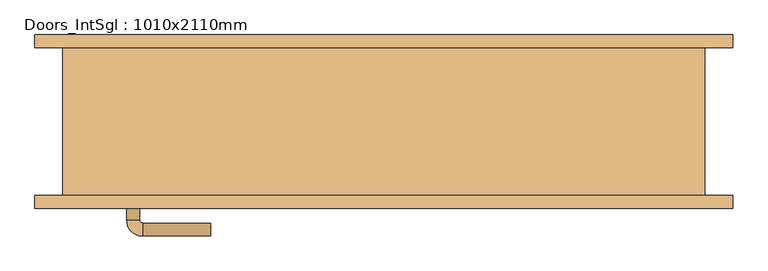
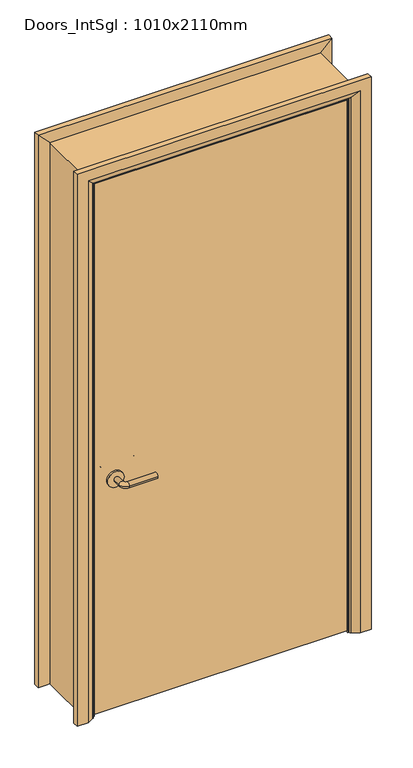
"""IFC4 building model written with IfcOpenShell, lengths in millimetres: door geometry, Doors_IntSgl : 1010x2110mm."""

from ifc_helpers import new_model, si_unit, point, frame, frame_2d, origin, place, context, project, spatial, polyline, circle_curve, ellipse_curve, trimmed, segment, composite_curve, outline, extrude, faceted_brep, source, transform, mapped, element, save
from ifc_brep_helpers import plane_surface, cylinder_surface, revolved_surface, advanced_brep


def doors_intsgl_1010x2110mm_2294229c(model_context):
    return source(origin(), model_context, "Body", "SolidModel", [
        advanced_brep(
        [(-398.0, -68.3, 900.0), (-378.0, -68.3, 900.0), (-398.0, -38.3, 900.0), (-378.0, -38.3, 900.0), (-373.0, -33.3, 900.0), (-373.0, -13.3, 900.0), (-268.0, -13.3, 900.0), (-268.0, -33.3, 900.0)],
        [
            (0, 1, circle_curve(frame((-388.0, -68.3, 900.0), z_axis=(0.0, -1.0, 0.0), x_axis=(1.0, 0.0, 0.0)), 10.0)),
            (1, 0, circle_curve(frame((-388.0, -68.3, 900.0), z_axis=(0.0, -1.0, 0.0), x_axis=(1.0, 0.0, 0.0)), 10.0)),
            (0, 2),
            (2, 3, circle_curve(frame((-388.0, -38.3, 900.0), z_axis=(0.0, -1.0, 0.0), x_axis=(1.0, 0.0, 0.0)), 10.0)),
            (3, 1),
            (3, 2, circle_curve(frame((-388.0, -38.3, 900.0), z_axis=(0.0, -1.0, 0.0), x_axis=(1.0, 0.0, 0.0)), 10.0)),
            (4, 3, circle_curve(frame((-373.0, -38.3, 900.0), z_axis=(0.0, 0.0, 1.0), x_axis=(-1.0, 0.0, 0.0)), 5.0)),
            (2, 5, circle_curve(frame((-373.0, -38.3, 900.0), z_axis=(0.0, 0.0, -1.0), x_axis=(-1.0, 0.0, 0.0)), 25.0)),
            (5, 4, circle_curve(frame((-373.0, -23.3, 900.0), z_axis=(-1.0, 0.0, 0.0), x_axis=(0.0, -1.0, 0.0)), 10.0)),
            (4, 5, circle_curve(frame((-373.0, -23.3, 900.0), z_axis=(-1.0, 0.0, 0.0), x_axis=(0.0, -1.0, 0.0)), 10.0)),
            (6, 7, circle_curve(frame((-268.0, -23.3, 900.0), z_axis=(1.0, 0.0, 0.0), x_axis=(0.0, -1.0, 0.0)), 10.0)),
            (7, 6, circle_curve(frame((-268.0, -23.3, 900.0), z_axis=(1.0, 0.0, 0.0), x_axis=(0.0, -1.0, 0.0)), 10.0)),
            (5, 6),
            (7, 4),
        ],
        [
            plane_surface(frame((-388.0, -68.3, 900.0), z_axis=(0.0, -1.0, 0.0), x_axis=(0.0, 0.0, 1.0))),
            cylinder_surface(frame((-388.0, -68.3, 900.0), z_axis=(0.0, -1.0, 0.0), x_axis=(1.0, 0.0, 0.0)), 10.0),
            revolved_surface(trimmed(ellipse_curve(frame((-388.0, -38.3, 900.0), z_axis=(0.0, -1.0, 0.0), x_axis=(1.0, 0.0, 0.0)), 10.0, 10.0), [point((-398.0, -38.3, 900.0))], [point((-378.0, -38.3, 900.0))], True, "CARTESIAN"), (-373.0, -38.3, 900.0), (0.0, 0.0, -1.0)),
            revolved_surface(trimmed(ellipse_curve(frame((-388.0, -38.3, 900.0), z_axis=(0.0, -1.0, 0.0), x_axis=(1.0, 0.0, 0.0)), 10.0, 10.0), [point((-378.0, -38.3, 900.0))], [point((-398.0, -38.3, 900.0))], True, "CARTESIAN"), (-373.0, -38.3, 900.0), (0.0, 0.0, -1.0)),
            plane_surface(frame((-268.0, -23.3, 900.0), z_axis=(1.0, 0.0, 0.0), x_axis=(0.0, 0.0, 1.0))),
            cylinder_surface(frame((-373.0, -23.3, 900.0), z_axis=(-1.0, 0.0, 0.0), x_axis=(0.0, -1.0, 0.0)), 10.0),
        ],
        [
            (0, [[1, 2]]),
            (1, [[-1, 3, 4, 5]]),
            (1, [[-2, -5, 6, -3]]),
            (2, [[7, -4, 8, 9]]),
            (3, [[-8, -6, -7, 10]]),
            (4, [[11, 12]]),
            (5, [[-9, 13, -12, 14]]),
            (5, [[-10, -14, -11, -13]]),
        ],
    ),
        extrude(outline(composite_curve([segment(trimmed(circle_curve(frame_2d((900.0, -390.5)), 30.0), [point((900.0, -420.5))], [point((900.0, -360.5))], False, "CARTESIAN"), True, "CONTINUOUS"), segment(trimmed(circle_curve(frame_2d((900.0, -390.5)), 30.0), [point((900.0, -360.5))], [point((900.0, -420.5))], False, "CARTESIAN"), True, "CONTINUOUS")], self_intersect=False)), frame((0.0, -76.3, 0.0), z_axis=(0.0, 1.0, 0.0), x_axis=(0.0, 0.0, 1.0)), (0.0, 0.0, 1.0), 8.0),
        advanced_brep(
        [(-398.0, -122.3, 900.0), (-378.0, -122.3, 900.0), (-378.0, -152.3, 900.0), (-398.0, -152.3, 900.0), (-373.0, -157.3, 900.0), (-373.0, -177.3, 900.0), (-268.0, -177.3, 900.0), (-268.0, -157.3, 900.0)],
        [
            (0, 1, circle_curve(frame((-388.0, -122.3, 900.0), z_axis=(0.0, 1.0, 0.0), x_axis=(1.0, 0.0, 0.0)), 10.0)),
            (1, 0, circle_curve(frame((-388.0, -122.3, 900.0), z_axis=(0.0, 1.0, 0.0), x_axis=(1.0, 0.0, 0.0)), 10.0)),
            (1, 2),
            (2, 3, circle_curve(frame((-388.0, -152.3, 900.0), z_axis=(0.0, 1.0, 0.0), x_axis=(1.0, 0.0, 0.0)), 10.0)),
            (3, 0),
            (3, 2, circle_curve(frame((-388.0, -152.3, 900.0), z_axis=(0.0, 1.0, 0.0), x_axis=(1.0, 0.0, 0.0)), 10.0)),
            (4, 5, circle_curve(frame((-373.0, -167.3, 900.0), z_axis=(-1.0, 0.0, 0.0), x_axis=(0.0, 1.0, 0.0)), 10.0)),
            (5, 3, circle_curve(frame((-373.0, -152.3, 900.0), z_axis=(0.0, 0.0, -1.0), x_axis=(-1.0, 0.0, 0.0)), 25.0)),
            (2, 4, circle_curve(frame((-373.0, -152.3, 900.0), z_axis=(0.0, 0.0, 1.0), x_axis=(-1.0, 0.0, 0.0)), 5.0)),
            (5, 4, circle_curve(frame((-373.0, -167.3, 900.0), z_axis=(-1.0, 0.0, 0.0), x_axis=(0.0, 1.0, 0.0)), 10.0)),
            (6, 7, circle_curve(frame((-268.0, -167.3, 900.0), z_axis=(1.0, 0.0, 0.0), x_axis=(0.0, 1.0, 0.0)), 10.0)),
            (7, 6, circle_curve(frame((-268.0, -167.3, 900.0), z_axis=(1.0, 0.0, 0.0), x_axis=(0.0, 1.0, 0.0)), 10.0)),
            (4, 7),
            (6, 5),
        ],
        [
            plane_surface(frame((-388.0, -122.3, 900.0), z_axis=(0.0, 1.0, 0.0), x_axis=(0.0, 0.0, 1.0))),
            cylinder_surface(frame((-388.0, -122.3, 900.0), z_axis=(0.0, 1.0, 0.0), x_axis=(1.0, 0.0, 0.0)), 10.0),
            revolved_surface(trimmed(ellipse_curve(frame((-388.0, -152.3, 900.0), z_axis=(0.0, -1.0, 0.0), x_axis=(1.0, 0.0, 0.0)), 10.0, 10.0), [point((-398.0, -152.3, 900.0))], [point((-378.0, -152.3, 900.0))], True, "CARTESIAN"), (-373.0, -152.3, 900.0), (0.0, 0.0, -1.0)),
            revolved_surface(trimmed(ellipse_curve(frame((-388.0, -152.3, 900.0), z_axis=(0.0, -1.0, 0.0), x_axis=(1.0, 0.0, 0.0)), 10.0, 10.0), [point((-378.0, -152.3, 900.0))], [point((-398.0, -152.3, 900.0))], True, "CARTESIAN"), (-373.0, -152.3, 900.0), (0.0, 0.0, -1.0)),
            plane_surface(frame((-268.0, -167.3, 900.0), z_axis=(1.0, 0.0, 0.0), x_axis=(0.0, 0.0, 1.0))),
            cylinder_surface(frame((-373.0, -167.3, 900.0), z_axis=(-1.0, 0.0, 0.0), x_axis=(0.0, 1.0, 0.0)), 10.0),
        ],
        [
            (0, [[1, 2]]),
            (1, [[3, 4, 5, -2]]),
            (1, [[-5, 6, -3, -1]]),
            (2, [[7, 8, -4, 9]]),
            (3, [[10, -9, -6, -8]]),
            (4, [[11, 12]]),
            (5, [[13, -11, 14, -7]]),
            (5, [[-14, -12, -13, -10]]),
        ],
    ),
        extrude(outline(composite_curve([segment(trimmed(circle_curve(frame_2d((900.0, -390.5)), 30.0), [point((900.0, -420.5))], [point((900.0, -360.5))], False, "CARTESIAN"), True, "CONTINUOUS"), segment(trimmed(circle_curve(frame_2d((900.0, -390.5)), 30.0), [point((900.0, -360.5))], [point((900.0, -420.5))], False, "CARTESIAN"), True, "CONTINUOUS")], self_intersect=False)), frame((0.0, -122.3, 0.0), z_axis=(0.0, 1.0, 0.0), x_axis=(0.0, 0.0, 1.0)), (0.0, 0.0, 1.0), 8.0),
        extrude(outline(polyline([(463.0, -76.3), (463.0, -114.3), (-463.0, -114.3), (-463.0, -76.3), (463.0, -76.3)])), frame((0.0, 0.0, 8.0), z_axis=(0.0, 0.0, 1.0), x_axis=(1.0, 0.0, 0.0)), (0.0, 0.0, 1.0), 2060.0),
        advanced_brep(
        [(540.0, -134.3, 0.0), (500.0, -134.3, 0.0), (474.0, -120.3, 0.0), (470.0, -114.3, 0.0), (540.0, -114.3, 0.0), (540.0, -114.3, 2145.0), (540.0, -134.3, 2145.0), (470.0, -114.3, 2075.0), (-470.0, -114.3, 2075.0), (-470.0, -114.3, 0.0), (-540.0, -114.3, 0.0), (-540.0, -114.3, 2145.0), (474.0, -120.3, 2079.0), (500.0, -134.3, 2105.0), (-540.0, -134.3, 2145.0), (-540.0, -134.3, 0.0), (-500.0, -134.3, 0.0), (-500.0, -134.3, 2105.0), (-474.0, -120.3, 2079.0), (-474.0, -120.3, 0.0)],
        [
            (0, 1),
            (1, 2),
            (2, 3, circle_curve(frame((478.0, -113.3, 0.0), z_axis=(0.0, 0.0, -1.0), x_axis=(1.0, 0.0, 0.0)), 8.0622577)),
            (3, 4),
            (4, 0),
            (4, 5),
            (5, 6),
            (6, 0),
            (3, 7),
            (7, 8),
            (8, 9),
            (9, 10),
            (10, 11),
            (11, 5),
            (2, 12),
            (12, 7, ellipse_curve(frame((478.0, -113.3, 2083.0), z_axis=(0.7071067811865475, 0.0, -0.7071067811865475), x_axis=(-0.7071067811865474, 0.0, -0.7071067811865476)), 11.4017543, 8.0622577)),
            (1, 13),
            (13, 12),
            (6, 14),
            (14, 15),
            (15, 16),
            (16, 17),
            (17, 13),
            (11, 14),
            (12, 18),
            (18, 8, ellipse_curve(frame((-478.0, -113.3, 2083.0), z_axis=(0.7071067811865475, 0.0, 0.7071067811865475), x_axis=(0.7071067811865476, 0.0, -0.7071067811865474)), 11.4017543, 8.0622577)),
            (17, 18),
            (15, 10),
            (9, 19, circle_curve(frame((-478.0, -113.3, 0.0), z_axis=(0.0, 0.0, -1.0), x_axis=(-1.0, 0.0, 0.0)), 8.0622577)),
            (19, 16),
            (18, 19),
        ],
        [
            plane_surface(frame((470.0, -114.3, 0.0), z_axis=(0.0, 0.0, -1.0), x_axis=(0.0, 1.0, 0.0))),
            plane_surface(frame((540.0, -134.3, 0.0), z_axis=(1.0, 0.0, 0.0), x_axis=(0.0, 0.0, 1.0))),
            plane_surface(frame((540.0, -114.3, 0.0), z_axis=(0.0, 1.0, 0.0), x_axis=(0.0, 0.0, 1.0))),
            cylinder_surface(frame((478.0, -113.3, 0.0), z_axis=(0.0, 0.0, -1.0), x_axis=(1.0, 0.0, 0.0)), 8.0622577),
            plane_surface(frame((474.0, -120.3, 0.0), z_axis=(-0.4740998230350126, -0.880471099922178, 0.0), x_axis=(0.0, 0.0, 1.0))),
            plane_surface(frame((500.0, -134.3, 0.0), z_axis=(0.0, -1.0, 0.0), x_axis=(0.0, 0.0, 1.0))),
            plane_surface(frame((540.0, -134.3, 2145.0), z_axis=(0.0, 0.0, 1.0), x_axis=(-1.0, 0.0, 0.0))),
            cylinder_surface(frame((470.0, -113.3, 2083.0), z_axis=(1.0, 0.0, 0.0), x_axis=(0.0, 0.0, 1.0)), 8.0622577),
            plane_surface(frame((474.0, -120.3, 2079.0), z_axis=(0.0, -0.8804710999221764, -0.4740998230350154), x_axis=(-1.0, 0.0, 0.0))),
            plane_surface(frame((-470.0, -114.3, 0.0), z_axis=(0.0, 0.0, -1.0), x_axis=(0.0, 1.0, 0.0))),
            plane_surface(frame((-540.0, -134.3, 2145.0), z_axis=(-1.0, 0.0, 0.0), x_axis=(0.0, 0.0, -1.0))),
            cylinder_surface(frame((-478.0, -113.3, 2075.0), z_axis=(0.0, 0.0, 1.0), x_axis=(-1.0, 0.0, 0.0)), 8.0622577),
            plane_surface(frame((-474.0, -120.3, 2079.0), z_axis=(0.47409982303501824, -0.8804710999221749, 0.0), x_axis=(0.0, 0.0, -1.0))),
        ],
        [
            (0, [[1, 2, 3, 4, 5]]),
            (1, [[6, 7, 8, -5]]),
            (2, [[9, 10, 11, 12, 13, 14, -6, -4]]),
            (3, [[15, 16, -9, -3]]),
            (4, [[17, 18, -15, -2]]),
            (5, [[-8, 19, 20, 21, 22, 23, -17, -1]]),
            (6, [[-14, 24, -19, -7]]),
            (7, [[25, 26, -10, -16]]),
            (8, [[-23, 27, -25, -18]]),
            (9, [[28, -12, 29, 30, -21]]),
            (10, [[-13, -28, -20, -24]]),
            (11, [[31, -29, -11, -26]]),
            (12, [[-22, -30, -31, -27]]),
        ],
    ),
        extrude(outline(polyline([(0.0, -446.0), (2051.0, -446.0), (2051.0, 446.0), (0.0, 446.0), (0.0, 465.0), (2070.0, 465.0), (2070.0, -465.0), (0.0, -465.0), (0.0, -446.0)])), frame((0.0, -74.3, 0.0), z_axis=(0.0, 1.0, 0.0), x_axis=(0.0, 0.0, 1.0)), (0.0, 0.0, 1.0), 32.0),
        advanced_brep(
        [(-540.0, 134.3, 0.0), (-500.0, 134.3, 0.0), (-474.0, 120.3, 0.0), (-470.0, 114.3, 0.0), (-540.0, 114.3, 0.0), (-540.0, 114.3, 2145.0), (-540.0, 134.3, 2145.0), (-470.0, 114.3, 2075.0), (-474.0, 120.3, 2079.0), (-500.0, 134.3, 2105.0), (540.0, 114.3, 2145.0), (540.0, 134.3, 2145.0), (470.0, 114.3, 2075.0), (474.0, 120.3, 2079.0), (500.0, 134.3, 2105.0), (540.0, 134.3, 0.0), (540.0, 114.3, 0.0), (470.0, 114.3, 0.0), (474.0, 120.3, 0.0), (500.0, 134.3, 0.0)],
        [
            (0, 1),
            (1, 2),
            (2, 3, circle_curve(frame((-478.0, 113.3, 0.0), z_axis=(0.0, 0.0, -1.0), x_axis=(-1.0, 0.0, 0.0)), 8.0622577)),
            (3, 4),
            (4, 0),
            (4, 5),
            (5, 6),
            (6, 0),
            (3, 7),
            (7, 5),
            (2, 8),
            (8, 7, ellipse_curve(frame((-478.0, 113.3, 2083.0), z_axis=(-0.7071067811865475, 0.0, -0.7071067811865475), x_axis=(0.7071067811865474, 0.0, -0.7071067811865476)), 11.4017543, 8.0622577)),
            (1, 9),
            (9, 8),
            (6, 9),
            (5, 10),
            (10, 11),
            (11, 6),
            (7, 12),
            (12, 10),
            (8, 13),
            (13, 12, ellipse_curve(frame((478.0, 113.3, 2083.0), z_axis=(-0.7071067811865475, 0.0, 0.7071067811865475), x_axis=(-0.7071067811865476, 0.0, -0.7071067811865474)), 11.4017543, 8.0622577)),
            (9, 14),
            (14, 13),
            (11, 14),
            (15, 16),
            (16, 17),
            (17, 18, circle_curve(frame((478.0, 113.3, 0.0), z_axis=(0.0, 0.0, -1.0), x_axis=(1.0, 0.0, 0.0)), 8.0622577)),
            (18, 19),
            (19, 15),
            (10, 16),
            (15, 11),
            (12, 17),
            (13, 18),
            (14, 19),
        ],
        [
            plane_surface(frame((-470.0, 187.1010989, 0.0), z_axis=(0.0, 0.0, -1.0), x_axis=(1.0, 0.0, 0.0))),
            plane_surface(frame((-540.0, 134.3, 0.0), z_axis=(-1.0, 0.0, 0.0), x_axis=(0.0, 0.0, 1.0))),
            plane_surface(frame((-540.0, 114.3, 0.0), z_axis=(0.0, -1.0, 0.0), x_axis=(0.0, 0.0, 1.0))),
            cylinder_surface(frame((-478.0, 113.3, 0.0), z_axis=(0.0, 0.0, -1.0), x_axis=(-1.0, 0.0, 0.0)), 8.0622577),
            plane_surface(frame((-474.0, 120.3, 0.0), z_axis=(0.4740998230350183, 0.8804710999221749, 0.0), x_axis=(0.0, 0.0, 1.0))),
            plane_surface(frame((-500.0, 134.3, 0.0), z_axis=(0.0, 1.0, 0.0), x_axis=(0.0, 0.0, 1.0))),
            plane_surface(frame((-540.0, 134.3, 2145.0), z_axis=(0.0, 0.0, 1.0), x_axis=(1.0, 0.0, 0.0))),
            plane_surface(frame((-540.0, 114.3, 2145.0), z_axis=(0.0, -1.0, 0.0), x_axis=(1.0, 0.0, 0.0))),
            cylinder_surface(frame((-470.0, 113.3, 2083.0), z_axis=(-1.0, 0.0, 0.0), x_axis=(0.0, 0.0, 1.0)), 8.0622577),
            plane_surface(frame((-474.0, 120.3, 2079.0), z_axis=(0.0, 0.8804710999221749, -0.4740998230350183), x_axis=(1.0, 0.0, 0.0))),
            plane_surface(frame((-500.0, 134.3, 2105.0), z_axis=(0.0, 1.0, 0.0), x_axis=(1.0, 0.0, 0.0))),
            plane_surface(frame((470.0, 187.1010989, 0.0), z_axis=(0.0, 0.0, -1.0), x_axis=(-1.0, 0.0, 0.0))),
            plane_surface(frame((540.0, 134.3, 2145.0), z_axis=(1.0, 0.0, 0.0), x_axis=(0.0, 0.0, -1.0))),
            plane_surface(frame((540.0, 114.3, 2145.0), z_axis=(0.0, -1.0, 0.0), x_axis=(0.0, 0.0, -1.0))),
            cylinder_surface(frame((478.0, 113.3, 2075.0), z_axis=(0.0, 0.0, 1.0), x_axis=(1.0, 0.0, 0.0)), 8.0622577),
            plane_surface(frame((474.0, 120.3, 2079.0), z_axis=(-0.4740998230350183, 0.8804710999221749, 0.0), x_axis=(0.0, 0.0, -1.0))),
            plane_surface(frame((500.0, 134.3, 2105.0), z_axis=(0.0, 1.0, 0.0), x_axis=(0.0, 0.0, -1.0))),
        ],
        [
            (0, [[1, 2, 3, 4, 5]]),
            (1, [[6, 7, 8, -5]]),
            (2, [[9, 10, -6, -4]]),
            (3, [[11, 12, -9, -3]]),
            (4, [[13, 14, -11, -2]]),
            (5, [[-8, 15, -13, -1]]),
            (6, [[16, 17, 18, -7]]),
            (7, [[19, 20, -16, -10]]),
            (8, [[21, 22, -19, -12]]),
            (9, [[23, 24, -21, -14]]),
            (10, [[-18, 25, -23, -15]]),
            (11, [[26, 27, 28, 29, 30]]),
            (12, [[31, -26, 32, -17]]),
            (13, [[33, -27, -31, -20]]),
            (14, [[34, -28, -33, -22]]),
            (15, [[35, -29, -34, -24]]),
            (16, [[-32, -30, -35, -25]]),
        ],
    ),
        faceted_brep([(-465.0, -114.3, 0.0), (-497.0, -114.3, 0.0), (-497.0, 114.3, 0.0), (-465.0, 114.3, 0.0), (-465.0, 114.3, 2070.0), (-465.0, -114.3, 2070.0), (-497.0, 114.3, 2102.0), (-497.0, -114.3, 2102.0), (465.0, 114.3, 2070.0), (465.0, -114.3, 2070.0), (497.0, 114.3, 2102.0), (497.0, -114.3, 2102.0), (465.0, -114.3, 0.0), (465.0, 114.3, 0.0), (497.0, 114.3, 0.0), (497.0, -114.3, 0.0)], [[[0, 1, 2, 3]], [[3, 4, 5, 0]], [[2, 6, 4, 3]], [[1, 7, 6, 2]], [[0, 5, 7, 1]], [[4, 8, 9, 5]], [[6, 10, 8, 4]], [[7, 11, 10, 6]], [[5, 9, 11, 7]], [[12, 13, 14, 15]], [[8, 13, 12, 9]], [[10, 14, 13, 8]], [[11, 15, 14, 10]], [[9, 12, 15, 11]]]),
    ])


if __name__ == "__main__":
    model = new_model("IFC4")
    model_context = context("Model", 3, world=origin())
    ifc_project = project(units=[si_unit("LENGTHUNIT", "METRE", prefix="MILLI")], contexts=[model_context])
    site = spatial("IfcSite", under=ifc_project)
    building = spatial("IfcBuilding", under=site)
    placement = place(None, origin())
    doors_intsgl_1010x2110mm_shape = doors_intsgl_1010x2110mm_2294229c(model_context)
    element("IfcDoor", 1, ObjectType="Doors_IntSgl : 1010x2110mm", at=placement, inside=building, context=model_context, shape_type="MappedRepresentation", body=[
        mapped(doors_intsgl_1010x2110mm_shape, transform((0.0, 0.0, 0.0), x_axis=(1.0, 0.0, 0.0), y_axis=(0.0, 1.0, 0.0), z_axis=(0.0, 0.0, 1.0))),
    ])
    save(model, "model.ifc")

# Revit data of these elements
# Type "Doors_IntSgl : 1010x2110mm"
#   Construction Type Id = "MDOOR"
#   Type Mark = "43"
#   Type Comments = "Internal Single"
#   Operation = "SingleSwingRight"
#   Manufacturer = "Revit"
#   Keynote = "L20"
#   Description = "Internal Single Door"
#   Analytic Construction = "Metal"
#   UnderCut = 8 mm
#   Tolerance = 2 mm
#   Thickness = 38 mm
#   Thermal Resistance (R) = 0.270117 (m²·K)/W
#   Structural Tolerance = 8 mm
#   StopDepth = 32 mm
#   Stop Thickness = 19 mm
#   Rough Width = 1010 mm
#   Rough Height = 2110 mm
#   Height to Top Lock Rail = 1000 mm
#   Heat Transfer Coefficient (U) = 3.7021 W/(m²·K)
#   Handle Z Distance = 900 mm
#   Handle X Distance = 75 mm
#   Frame Thickness = 32 mm
#   Door Panel Width = 926 mm
#   Door Panel Thickness = 38 mm
#   Door Panel Offset = 0 mm
#   Height = 2110 mm
#   Width = 1010 mm
#   Door Panel Height = 2060 mm
#   Architrave Setback = 5 mm
#   Define Thermal Properties by = 1
#   Vis - Ironmongery = yes
#   Material Ironmongery = Door - Handle
#   Material Frame = Door - Frame/Mullion (1)
#   Material Door = Door - Panel
#   Material Architrave = Door - Architrave
#   Visual Light Transmittance = 0
#   Solar Heat Gain Coefficient = 0
#   Function = (empty or 0)
#   Wall Closure = (empty or 0)
# Element 1 (IfcDoor, "Doors_IntSgl : 1010x2110mm")
#   Materials on its faces: "Door - Architrave", "Door - Handle", "Door - Frame/Mullion (1)", "Door - Panel"
# Materials
#   "Door - Handle": colour RGB 0 0 0, transparency 0, Keynote = "P21", Cost = 0
#   "Door - Frame/Mullion (1)": class "Wood", colour RGB 212 179 113, transparency 0, Keynote = "L20", Cost = 0
#   "Door - Panel": class "Wood", colour RGB 210 159 95, transparency 0, Keynote = "L20", Cost = 0
#   "Door - Architrave": class "Wood", colour RGB 154 90 5, transparency 0, Keynote = "P20", Cost = 0
